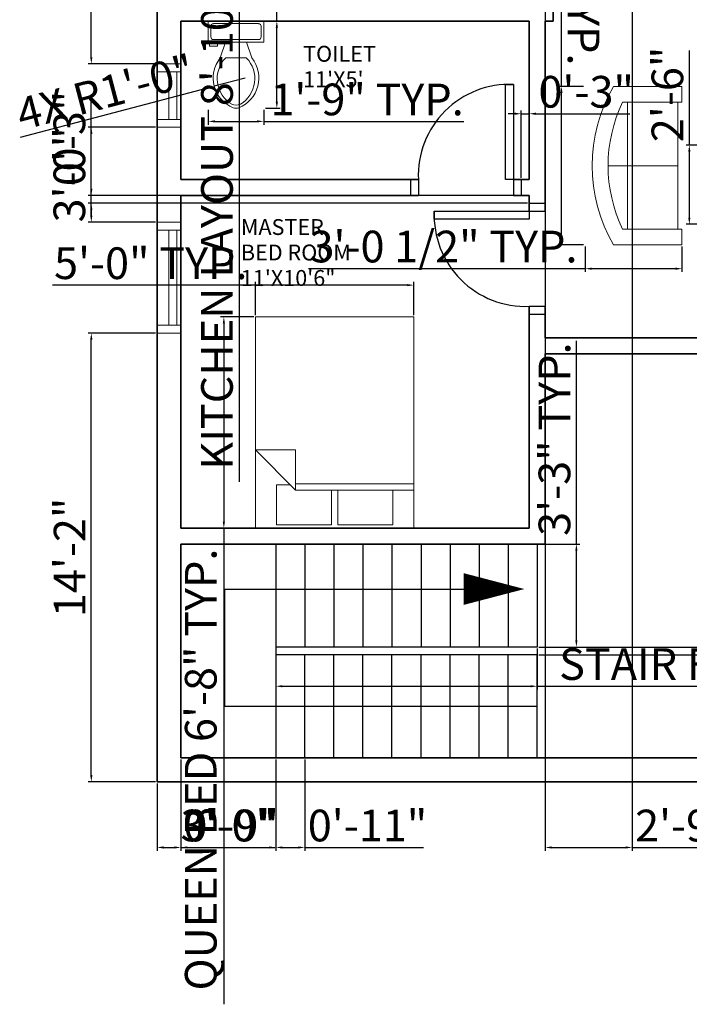
# Model space of a CAD drawing. Units: inches. Extents: x 2330 to 2931, y 514 to 1098.
# Tile 1 of 4: x 2330 to 2583, y 514 to 887. Entities that reach past the tile are written whole.
import ezdxf

# ---------------------------------------------------------------- set-up
doc = ezdxf.new("R2010")
doc.units = ezdxf.units.IN
for name, color, linetype, lineweight in [('A-ANNO-DIMS', 2, 'Continuous', 18), ('A-AREA-IDEN', 7, 'Continuous', 18), ('A-DOOR', 3, 'Continuous', 25), ('A-FLOR-FIXT', 9, 'Continuous', 18), ('A-FLOR-STRS', 7, 'Continuous', 25), ('A-FURN', 8, 'Continuous', 18), ('A-GLAZ', 4, 'Continuous', 18), ('A-WALL', 7, 'Continuous', 35)]:
    doc.layers.add(name, color=color, linetype=linetype, lineweight=lineweight)
doc.styles.get("Standard").update_dxf_attribs({"font": 'arial.ttf'})
doc.dimstyles.new('ISO-25', dxfattribs={"dimtxt": 12, "dimasz": 2.5, "dimexe": 1.25, "dimexo": 0.625, "dimtad": 1, "dimdec": 1, "dimlunit": 3, "dimtxsty": 'Standard', "dimcen": 2.5, "dimadec": 0, "dimazin": 0, "dimtfac": 1, "dimtdec": 1, "dimtmove": 0, "dimatfit": 3, "dimfxl": 1, "dimarcsym": 0})

# ---------------------------------------------------------------- blocks, each defined once
blk = doc.blocks.new('Toilet - top')
for p, q in [((9.5, -6), (9.5, -2)), ((-10, -8.5), (-8, -8.5)), ((-10, -9.5), (-10, -8.5)), ((-7, -9.5), (-10, -9.5)), ((-8, -8.5), (-8, -8)), ((-7, -8), (-7, -9.5)), ((-4, -8), (-6, -14)), ((4, -8), (6, -14)), ((4, -14), (-4, -14))]:
    blk.add_line(p, q)
blk.add_lwpolyline([(10.5, -8), (10.5, 0), (-10.5, 0), (-10.5, -8)], close=True)
for points in [[(-9.5, -2), (-9.5, -6)], [(8.5, -1), (-8.5, -1)], [(-8.5, -7), (8.5, -7)]]:
    blk.add_lwpolyline(points)
for centre, radius, start, end in [((-8.62, -1.88), 0.884, 81.8699, 188.1301), ((8.62, -1.88), 0.884, 351.8699, 98.1301), ((-8.62, -6.12), 0.884, 171.8699, 278.1301), ((8.62, -6.12), 0.884, 261.8699, 8.1301), ((3.52, -21.58), 12.17, 141.4691, 247.9714), ((4.2, -21.82), 11.33, 136.3677, 238.9468), ((-3.52, -21.58), 12.17, 292.0284, 38.5307), ((-4.2, -21.82), 11.33, 301.053, 43.6321), ((0, -27.88), 4, 245.7318, 294.2682), ((0, -29), 4, 254.8605, 285.1395)]:
    blk.add_arc(centre, radius, start, end)
blk = doc.blocks.new('Bed - Queen')
for p, q in [((0, -80.00003), (0, 0)), ((0, 0), (59.99999, 0)), ((59.99999, 0), (59.99999, -80.00003)), ((7.99999, -1.2), (28.79998, -1.2)), ((7.99999, -14.4), (7.99999, -1.2)), ((28.79998, -1.2), (28.79998, -14.4)), ((31.19999, -1.2), (51.99999, -1.2)), ((31.19999, -14.4), (31.19999, -1.2)), ((51.99999, -1.2), (51.99999, -16.4)), ((0, -14.4), (44.8, -14.4)), ((59.99999, -29.6), (44.8, -14.4)), ((44.8, -14.4), (44.8, -29.6)), ((44.8, -16.8), (0, -16.8)), ((51.99999, -16.4), (46.79936, -16.4)), ((44.8, -29.6), (59.99999, -29.6)), ((59.99999, -80.00003), (0, -80.00003))]:
    blk.add_line(p, q)
blk = doc.blocks.new('Sofa - Roundback Loveseat 5 ft.')
for p, q in [((0, -32.44198), (0, -5.99998)), ((-24, -33.99998), (-24, -11.46958)), ((-23.9998, -13.38178), (23.99986, -13.38178)), ((24.00004, -33.99998), (24.00004, -11.46958)), ((-24, -32.44198), (24.00004, -32.44198))]:
    blk.add_line(p, q)
for points in [[(-24, -33.99998), (-30, -33.99998), (-30, -7.99998)], [(30.00004, -7.99998), (30.00004, -33.99998), (24.00004, -33.99998)]]:
    blk.add_lwpolyline(points)
for centre, radius, start, end in [((0, -60.24998), 60.24998, 60.13715, 119.8628), ((0, -61.38438), 55.38444, 64.32083, 115.6792)]:
    blk.add_arc(centre, radius, start, end)
blk = doc.blocks.new('DOOR-SWING-36IN')
for p, q in [((0, 6), (0, 0)), ((3, 6), (3, 0)), ((39, 6), (39, 0)), ((42, 6), (42, 0))]:
    blk.add_line(p, q)
blk.add_lwpolyline([(39, 6), (36, 6), (36, 42), (39, 42)], close=True)
blk.add_arc((37.5, 7.5), 34.53, 87.5104, 182.4896)
blk = doc.blocks.new('WIN-36IN')
for p, q in [((0, 9), (0, 0)), ((39, 9), (3, 9)), ((3, 9), (3, 0)), ((39, 0), (39, 9)), ((42, 0), (42, 9)), ((3, 4.5), (39, 4.5)), ((3, 1.5), (39, 1.5)), ((3, 0), (39, 0))]:
    blk.add_line(p, q)
blk = doc.blocks.new('WIN-18IN')
for p, q in [((0, 9), (0, 0)), ((21, 9), (3, 9)), ((3, 9), (3, 0)), ((21, 0), (21, 9)), ((24, 0), (24, 9)), ((3, 4.5), (21, 4.5)), ((3, 1.5), (21, 1.5)), ((3, 0), (21, 0))]:
    blk.add_line(p, q)
blk = doc.blocks.new('STAIR-FLIGHT-9-TREAD')
for p, q in [((11, 39), (11, 0)), ((22, 39), (22, 0)), ((33, 39), (33, 0)), ((44, 39), (44, 0)), ((55, 39), (55, 0)), ((66, 39), (66, 0)), ((77, 39), (77, 0)), ((88, 39), (88, 0)), ((99, 39), (99, 0)), ((99, 0), (0, 0))]:
    blk.add_line(p, q)
blk = doc.blocks.new('*D21')
at = {"layer": 'A-ANNO-DIMS', "color": 0, "lineweight": -2, "transparency": 16777216}
for p, q in [((2418.49, 774.47), (2405.87, 774.47)), ((2407.12, 771.97), (2407.12, 696.97)), ((2418.49, 694.47), (2405.87, 694.47)), ((2407.12, 694.47), (2407.12, 514.2))]:
    blk.add_line(p, q, dxfattribs=at)
at = {"layer": 'A-ANNO-DIMS', "color": 0, "transparency": 16777216}
for points in [[(2406.7, 771.97), (2407.53, 771.97), (2407.12, 774.47)], [(2406.7, 696.97), (2407.53, 696.97), (2407.12, 694.47)]]:
    blk.add_solid(points, dxfattribs=at)
at = {"layer": 'Defpoints', "color": 0, "transparency": 16777216}
for p in [(2419.12, 774.47), (2407.12, 694.47), (2419.12, 694.47)]:
    blk.add_point(p, dxfattribs=at)
at = {"layer": 'A-ANNO-DIMS', "color": 0, "transparency": 16777216, "insert": (2399.92, 603.09), "char_height": 12, "attachment_point": 5, "rotation": 90}
blk.add_mtext('QUEEN BED 6\'-8" TYP.', dxfattribs=at)
blk = doc.blocks.new('*D22')
at = {"layer": 'A-ANNO-DIMS', "color": 0, "lineweight": -2, "transparency": 16777216}
for p, q in [((2419.12, 775.1), (2419.12, 787.72)), ((2479.12, 775.1), (2479.12, 787.72)), ((2419.12, 786.47), (2342.22, 786.47)), ((2476.62, 786.47), (2421.62, 786.47))]:
    blk.add_line(p, q, dxfattribs=at)
at = {"layer": 'A-ANNO-DIMS', "color": 0, "transparency": 16777216}
for points in [[(2421.62, 786.89), (2421.62, 786.06), (2419.12, 786.47)], [(2476.62, 786.89), (2476.62, 786.06), (2479.12, 786.47)]]:
    blk.add_solid(points, dxfattribs=at)
at = {"layer": 'Defpoints', "color": 0, "transparency": 16777216}
for p in [(2419.12, 786.47), (2419.12, 774.47), (2479.12, 774.47)]:
    blk.add_point(p, dxfattribs=at)
at = {"layer": 'A-ANNO-DIMS', "color": 0, "transparency": 16777216, "insert": (2379.42, 793.22), "char_height": 12, "attachment_point": 5}
blk.add_mtext('5\'-0" TYP.', dxfattribs=at)
blk = doc.blocks.new('*D23')
at = {"layer": 'A-ANNO-DIMS', "color": 0, "lineweight": -2, "transparency": 16777216}
for p, q in [((2427.19, 886.47), (2427.19, 996.45)), ((2422.86, 886.47), (2428.44, 886.47)), ((2427.19, 855.93), (2427.19, 883.97)), ((2422.86, 853.43), (2428.44, 853.43))]:
    blk.add_line(p, q, dxfattribs=at)
at = {"layer": 'A-ANNO-DIMS', "color": 0, "transparency": 16777216}
for points in [[(2426.77, 883.97), (2427.61, 883.97), (2427.19, 886.47)], [(2426.77, 855.93), (2427.61, 855.93), (2427.19, 853.43)]]:
    blk.add_solid(points, dxfattribs=at)
at = {"layer": 'Defpoints', "color": 0, "transparency": 16777216}
for p in [(2422.23, 886.47), (2427.19, 886.47), (2422.23, 853.43)]:
    blk.add_point(p, dxfattribs=at)
at = {"layer": 'A-ANNO-DIMS', "color": 0, "transparency": 16777216, "insert": (2420.36, 942.71), "char_height": 12, "attachment_point": 5, "rotation": 90}
blk.add_mtext('WC 2\'-9" TYP.', dxfattribs=at)
blk = doc.blocks.new('*D24')
at = {"layer": 'A-ANNO-DIMS', "color": 0, "lineweight": -2, "transparency": 16777216}
for p, q in [((2401.23, 852.8), (2401.23, 847.22)), ((2422.23, 852.8), (2422.23, 847.22)), ((2403.73, 848.47), (2419.73, 848.47)), ((2422.23, 848.47), (2498, 848.47))]:
    blk.add_line(p, q, dxfattribs=at)
at = {"layer": 'A-ANNO-DIMS', "color": 0, "transparency": 16777216}
for points in [[(2403.73, 848.89), (2403.73, 848.05), (2401.23, 848.47)], [(2419.73, 848.89), (2419.73, 848.05), (2422.23, 848.47)]]:
    blk.add_solid(points, dxfattribs=at)
at = {"layer": 'Defpoints', "color": 0, "transparency": 16777216}
for p in [(2401.23, 853.43), (2422.23, 853.43), (2422.23, 848.47)]:
    blk.add_point(p, dxfattribs=at)
at = {"layer": 'A-ANNO-DIMS', "color": 0, "transparency": 16777216, "insert": (2461.36, 855.22), "char_height": 12, "attachment_point": 5}
blk.add_mtext('1\'-9" TYP.', dxfattribs=at)
blk = doc.blocks.new('*D25')
at = {"layer": 'A-ANNO-DIMS', "color": 0, "lineweight": -2, "transparency": 16777216}
for p, q in [((2535, 861.7), (2535, 1031.23)), ((2543.37, 861.7), (2533.75, 861.7)), ((2535, 804.2), (2535, 859.2)), ((2543.37, 801.7), (2533.75, 801.7))]:
    blk.add_line(p, q, dxfattribs=at)
at = {"layer": 'A-ANNO-DIMS', "color": 0, "transparency": 16777216}
for points in [[(2535.41, 859.2), (2534.58, 859.2), (2535, 861.7)], [(2535.41, 804.2), (2534.58, 804.2), (2535, 801.7)]]:
    blk.add_solid(points, dxfattribs=at)
at = {"layer": 'Defpoints', "color": 0, "transparency": 16777216}
for p in [(2535, 861.7), (2544, 861.7), (2544, 801.7)]:
    blk.add_point(p, dxfattribs=at)
at = {"layer": 'A-ANNO-DIMS', "color": 0, "transparency": 16777216, "insert": (2541.83, 947.72), "char_height": 12, "attachment_point": 5, "rotation": 270.0001}
blk.add_mtext('LOVESEAT 5\'-0" TYP.', dxfattribs=at)
blk = doc.blocks.new('*D26')
at = {"layer": 'A-ANNO-DIMS', "color": 0, "lineweight": -2, "transparency": 16777216}
for p, q in [((2544, 801.08), (2544, 791.45)), ((2580.66, 801.08), (2580.66, 791.45)), ((2544, 792.7), (2439.15, 792.7)), ((2578.16, 792.7), (2546.5, 792.7))]:
    blk.add_line(p, q, dxfattribs=at)
at = {"layer": 'A-ANNO-DIMS', "color": 0, "transparency": 16777216}
for points in [[(2546.5, 793.12), (2546.5, 792.28), (2544, 792.7)], [(2578.16, 793.12), (2578.16, 792.28), (2580.66, 792.7)]]:
    blk.add_solid(points, dxfattribs=at)
at = {"layer": 'Defpoints', "color": 0, "transparency": 16777216}
for p in [(2544, 801.7), (2580.66, 801.7), (2544, 792.7)]:
    blk.add_point(p, dxfattribs=at)
at = {"layer": 'A-ANNO-DIMS', "color": 0, "transparency": 16777216, "insert": (2490.32, 799.53), "char_height": 12, "attachment_point": 5, "rotation": 0.0001}
blk.add_mtext('3\'-0 1/2" TYP.', dxfattribs=at)
blk = doc.blocks.new('*D29')
at = {"layer": 'A-ANNO-DIMS', "color": 0, "lineweight": -2, "transparency": 16777216}
for p, q in [((2426.8, 648.85), (2426.8, 633.37)), ((2525.8, 648.85), (2525.8, 633.37)), ((2429.3, 634.62), (2523.3, 634.62)), ((2525.8, 634.62), (2720.93, 634.62))]:
    blk.add_line(p, q, dxfattribs=at)
at = {"layer": 'A-ANNO-DIMS', "color": 0, "transparency": 16777216}
for points in [[(2429.3, 635.04), (2429.3, 634.21), (2426.8, 634.62)], [(2523.3, 635.04), (2523.3, 634.21), (2525.8, 634.62)]]:
    blk.add_solid(points, dxfattribs=at)
at = {"layer": 'Defpoints', "color": 0, "transparency": 16777216}
for p in [(2426.8, 649.47), (2525.8, 649.47), (2525.8, 634.62)]:
    blk.add_point(p, dxfattribs=at)
at = {"layer": 'A-ANNO-DIMS', "color": 0, "transparency": 16777216, "insert": (2624.62, 641.46), "char_height": 12, "attachment_point": 5}
blk.add_mtext('STAIR FLIGHT 8\'-3" TYP.', dxfattribs=at)
blk = doc.blocks.new('*D30')
at = {"layer": 'A-ANNO-DIMS', "color": 0, "lineweight": -2, "transparency": 16777216}
for p, q in [((2540.65, 688.47), (2540.65, 765.36)), ((2526.43, 688.47), (2541.9, 688.47)), ((2540.65, 651.97), (2540.65, 685.97)), ((2526.43, 649.47), (2541.9, 649.47))]:
    blk.add_line(p, q, dxfattribs=at)
at = {"layer": 'A-ANNO-DIMS', "color": 0, "transparency": 16777216}
for points in [[(2540.24, 685.97), (2541.07, 685.97), (2540.65, 688.47)], [(2540.24, 651.97), (2541.07, 651.97), (2540.65, 649.47)]]:
    blk.add_solid(points, dxfattribs=at)
at = {"layer": 'Defpoints', "color": 0, "transparency": 16777216}
for p in [(2525.8, 688.47), (2540.65, 688.47), (2525.8, 649.47)]:
    blk.add_point(p, dxfattribs=at)
at = {"layer": 'A-ANNO-DIMS', "color": 0, "transparency": 16777216, "insert": (2533.9, 728.17), "char_height": 12, "attachment_point": 5, "rotation": 90}
blk.add_mtext('3\'-3" TYP.', dxfattribs=at)
blk = doc.blocks.new('*D31')
at = {"layer": 'A-ANNO-DIMS', "color": 0, "lineweight": -2, "transparency": 16777216}
for p, q in [((2428.18, 1012.47), (2411.65, 1012.47)), ((2412.9, 1009.97), (2412.9, 908.97)), ((2428.18, 906.47), (2411.65, 906.47)), ((2412.9, 906.47), (2412.9, 712.06))]:
    blk.add_line(p, q, dxfattribs=at)
at = {"layer": 'A-ANNO-DIMS', "color": 0, "transparency": 16777216}
for points in [[(2412.49, 1009.97), (2413.32, 1009.97), (2412.9, 1012.47)], [(2412.49, 908.97), (2413.32, 908.97), (2412.9, 906.47)]]:
    blk.add_solid(points, dxfattribs=at)
at = {"layer": 'Defpoints', "color": 0, "transparency": 16777216}
for p in [(2428.8, 1012.47), (2412.9, 906.47), (2428.8, 906.47)]:
    blk.add_point(p, dxfattribs=at)
at = {"layer": 'A-ANNO-DIMS', "color": 0, "transparency": 16777216, "insert": (2406.07, 808.02), "char_height": 12, "attachment_point": 5, "rotation": 90}
blk.add_mtext('KITCHEN LAYOUT 8\'-10"', dxfattribs=at)
blk = doc.blocks.new('*D34')
at = {"layer": 'A-ANNO-DIMS', "color": 0, "lineweight": -2, "transparency": 16777216}
for p, q in [((2583.44, 839.51), (2583.44, 875.36)), ((2591.82, 839.51), (2582.19, 839.51)), ((2583.44, 812.01), (2583.44, 837.01)), ((2591.82, 809.51), (2582.19, 809.51))]:
    blk.add_line(p, q, dxfattribs=at)
at = {"layer": 'A-ANNO-DIMS', "color": 0, "transparency": 16777216}
for points in [[(2583.03, 837.01), (2583.86, 837.01), (2583.44, 839.51)], [(2583.03, 812.01), (2583.86, 812.01), (2583.44, 809.51)]]:
    blk.add_solid(points, dxfattribs=at)
at = {"layer": 'Defpoints', "color": 0, "transparency": 16777216}
for p in [(2583.44, 839.51), (2592.44, 839.51), (2592.44, 809.51)]:
    blk.add_point(p, dxfattribs=at)
at = {"layer": 'A-ANNO-DIMS', "color": 0, "transparency": 16777216, "insert": (2576.69, 858.69), "char_height": 12, "attachment_point": 5, "rotation": 90}
blk.add_mtext('2\'-6"', dxfattribs=at)
blk = doc.blocks.new('*D42')
at = {"layer": 'A-ANNO-DIMS', "color": 0, "lineweight": -2, "transparency": 16777216}
for p, q in [((2381.18, 768.34), (2355.66, 768.34)), ((2356.91, 600.97), (2356.91, 765.84)), ((2381.18, 598.47), (2355.66, 598.47))]:
    blk.add_line(p, q, dxfattribs=at)
at = {"layer": 'A-ANNO-DIMS', "color": 0, "transparency": 16777216}
for points in [[(2356.49, 765.84), (2357.33, 765.84), (2356.91, 768.34)], [(2356.49, 600.97), (2357.33, 600.97), (2356.91, 598.47)]]:
    blk.add_solid(points, dxfattribs=at)
at = {"layer": 'Defpoints', "color": 0, "transparency": 16777216}
for p in [(2356.91, 768.34), (2381.8, 768.34), (2381.8, 598.47)]:
    blk.add_point(p, dxfattribs=at)
at = {"layer": 'A-ANNO-DIMS', "color": 0, "transparency": 16777216, "insert": (2350.26, 683.41), "char_height": 12, "attachment_point": 5, "rotation": 90}
blk.add_mtext('14\'-2"', dxfattribs=at)
blk = doc.blocks.new('*D43')
at = {"layer": 'A-ANNO-DIMS', "color": 0, "lineweight": -2, "transparency": 16777216}
for p, q in [((2381.18, 846.23), (2355.66, 846.23)), ((2356.91, 812.84), (2356.91, 843.73)), ((2381.18, 810.34), (2355.66, 810.34))]:
    blk.add_line(p, q, dxfattribs=at)
at = {"layer": 'A-ANNO-DIMS', "color": 0, "transparency": 16777216}
for points in [[(2356.49, 843.73), (2357.33, 843.73), (2356.91, 846.23)], [(2356.49, 812.84), (2357.33, 812.84), (2356.91, 810.34)]]:
    blk.add_solid(points, dxfattribs=at)
at = {"layer": 'Defpoints', "color": 0, "transparency": 16777216}
for p in [(2356.91, 846.23), (2381.8, 846.23), (2381.8, 810.34)]:
    blk.add_point(p, dxfattribs=at)
at = {"layer": 'A-ANNO-DIMS', "color": 0, "transparency": 16777216, "insert": (2350.15, 828.29), "char_height": 12, "attachment_point": 5, "rotation": 90}
blk.add_mtext('3\'-0"', dxfattribs=at)
blk = doc.blocks.new('*D44')
at = {"layer": 'A-ANNO-DIMS', "color": 0, "lineweight": -2, "transparency": 16777216}
for p, q in [((2356.91, 892.47), (2356.91, 936.31)), ((2390.18, 892.47), (2355.66, 892.47)), ((2356.91, 872.73), (2356.91, 889.97)), ((2381.18, 870.23), (2355.66, 870.23))]:
    blk.add_line(p, q, dxfattribs=at)
at = {"layer": 'A-ANNO-DIMS', "color": 0, "transparency": 16777216}
for points in [[(2356.49, 889.97), (2357.33, 889.97), (2356.91, 892.47)], [(2356.49, 872.73), (2357.33, 872.73), (2356.91, 870.23)]]:
    blk.add_solid(points, dxfattribs=at)
at = {"layer": 'Defpoints', "color": 0, "transparency": 16777216}
for p in [(2356.91, 892.47), (2390.8, 892.47), (2381.8, 870.23)]:
    blk.add_point(p, dxfattribs=at)
at = {"layer": 'A-ANNO-DIMS', "color": 0, "transparency": 16777216, "insert": (2350.16, 915.64), "char_height": 12, "attachment_point": 5, "rotation": 90}
blk.add_mtext('1\'-10"', dxfattribs=at)
blk = doc.blocks.new('*D48')
at = {"layer": 'A-ANNO-DIMS', "color": 0, "lineweight": -2, "transparency": 16777216}
for p, q in [((2390.8, 606.85), (2390.8, 572.33)), ((2426.8, 606.85), (2426.8, 572.33)), ((2393.3, 573.58), (2424.3, 573.58))]:
    blk.add_line(p, q, dxfattribs=at)
at = {"layer": 'A-ANNO-DIMS', "color": 0, "transparency": 16777216}
for points in [[(2393.3, 574), (2393.3, 573.16), (2390.8, 573.58)], [(2424.3, 574), (2424.3, 573.16), (2426.8, 573.58)]]:
    blk.add_solid(points, dxfattribs=at)
at = {"layer": 'Defpoints', "color": 0, "transparency": 16777216}
for p in [(2390.8, 607.47), (2426.8, 607.47), (2426.8, 573.58)]:
    blk.add_point(p, dxfattribs=at)
at = {"layer": 'A-ANNO-DIMS', "color": 0, "transparency": 16777216, "insert": (2408.8, 580.34), "char_height": 12, "attachment_point": 5}
blk.add_mtext('3\'-0"', dxfattribs=at)
blk = doc.blocks.new('*D49')
at = {"layer": 'A-ANNO-DIMS', "color": 0, "lineweight": -2, "transparency": 16777216}
for p, q in [((2390.8, 606.85), (2390.8, 572.33)), ((2381.8, 597.85), (2381.8, 572.33)), ((2384.3, 573.58), (2388.3, 573.58)), ((2390.8, 573.58), (2426.45, 573.58))]:
    blk.add_line(p, q, dxfattribs=at)
at = {"layer": 'A-ANNO-DIMS', "color": 0, "transparency": 16777216}
for points in [[(2384.3, 574), (2384.3, 573.16), (2381.8, 573.58)], [(2388.3, 574), (2388.3, 573.16), (2390.8, 573.58)]]:
    blk.add_solid(points, dxfattribs=at)
at = {"layer": 'Defpoints', "color": 0, "transparency": 16777216}
for p in [(2390.8, 607.47), (2381.8, 598.47), (2390.8, 573.58)]:
    blk.add_point(p, dxfattribs=at)
at = {"layer": 'A-ANNO-DIMS', "color": 0, "transparency": 16777216, "insert": (2409.88, 580.33), "char_height": 12, "attachment_point": 5}
blk.add_mtext('0\'-9"', dxfattribs=at)
blk = doc.blocks.new('*D50')
at = {"layer": 'A-ANNO-DIMS', "color": 0, "lineweight": -2, "transparency": 16777216}
for p, q in [((2426.8, 606.85), (2426.8, 572.33)), ((2437.8, 606.85), (2437.8, 572.33)), ((2429.3, 573.58), (2435.3, 573.58)), ((2437.8, 573.58), (2482.78, 573.58))]:
    blk.add_line(p, q, dxfattribs=at)
at = {"layer": 'A-ANNO-DIMS', "color": 0, "transparency": 16777216}
for points in [[(2429.3, 574), (2429.3, 573.16), (2426.8, 573.58)], [(2435.3, 574), (2435.3, 573.16), (2437.8, 573.58)]]:
    blk.add_solid(points, dxfattribs=at)
at = {"layer": 'Defpoints', "color": 0, "transparency": 16777216}
for p in [(2426.8, 607.47), (2437.8, 607.47), (2437.8, 573.58)]:
    blk.add_point(p, dxfattribs=at)
at = {"layer": 'A-ANNO-DIMS', "color": 0, "transparency": 16777216, "insert": (2461.54, 580.33), "char_height": 12, "attachment_point": 5}
blk.add_mtext('0\'-11"', dxfattribs=at)
blk = doc.blocks.new('*D52')
at = {"layer": 'A-ANNO-DIMS', "color": 0, "lineweight": -2, "transparency": 16777216}
for p, q in [((2778.7, 651.97), (2778.7, 687.62)), ((2526.43, 649.47), (2779.95, 649.47)), ((2778.7, 646.47), (2778.7, 649.47)), ((2526.43, 646.47), (2779.95, 646.47)), ((2778.7, 643.97), (2778.7, 641.47))]:
    blk.add_line(p, q, dxfattribs=at)
at = {"layer": 'A-ANNO-DIMS', "color": 0, "transparency": 16777216}
for points in [[(2778.28, 651.97), (2779.11, 651.97), (2778.7, 649.47)], [(2778.28, 643.97), (2779.11, 643.97), (2778.7, 646.47)]]:
    blk.add_solid(points, dxfattribs=at)
at = {"layer": 'Defpoints', "color": 0, "transparency": 16777216}
for p in [(2525.8, 649.47), (2778.7, 649.47), (2525.8, 646.47)]:
    blk.add_point(p, dxfattribs=at)
at = {"layer": 'A-ANNO-DIMS', "color": 0, "transparency": 16777216, "insert": (2771.94, 671.05), "char_height": 12, "attachment_point": 5, "rotation": 90}
blk.add_mtext('0\'-3"', dxfattribs=at)
blk = doc.blocks.new('*D54')
at = {"layer": 'A-ANNO-DIMS', "color": 0, "lineweight": -2, "transparency": 16777216}
for p, q in [((2517.3, 851.36), (2514.8, 851.36)), ((2519.8, 827.1), (2519.8, 852.61)), ((2519.8, 851.36), (2522.8, 851.36)), ((2522.8, 827.1), (2522.8, 852.61)), ((2525.3, 851.36), (2560.95, 851.36))]:
    blk.add_line(p, q, dxfattribs=at)
at = {"layer": 'A-ANNO-DIMS', "color": 0, "transparency": 16777216}
for points in [[(2517.3, 851.78), (2517.3, 850.95), (2519.8, 851.36)], [(2525.3, 851.78), (2525.3, 850.95), (2522.8, 851.36)]]:
    blk.add_solid(points, dxfattribs=at)
at = {"layer": 'Defpoints', "color": 0, "transparency": 16777216}
for p in [(2522.8, 851.36), (2519.8, 826.47), (2522.8, 826.47)]:
    blk.add_point(p, dxfattribs=at)
at = {"layer": 'A-ANNO-DIMS', "color": 0, "transparency": 16777216, "insert": (2544.38, 858.12), "char_height": 12, "attachment_point": 5}
blk.add_mtext('0\'-3"', dxfattribs=at)
blk = doc.blocks.new('*D55')
at = {"layer": 'A-ANNO-DIMS', "color": 0, "lineweight": -2, "transparency": 16777216}
for p, q in [((2356.91, 822.97), (2356.91, 858.62)), ((2522.18, 820.47), (2355.66, 820.47)), ((2356.91, 817.47), (2356.91, 820.47)), ((2522.18, 817.47), (2355.66, 817.47)), ((2356.91, 814.97), (2356.91, 812.47))]:
    blk.add_line(p, q, dxfattribs=at)
at = {"layer": 'A-ANNO-DIMS', "color": 0, "transparency": 16777216}
for points in [[(2356.49, 822.97), (2357.33, 822.97), (2356.91, 820.47)], [(2356.49, 814.97), (2357.33, 814.97), (2356.91, 817.47)]]:
    blk.add_solid(points, dxfattribs=at)
at = {"layer": 'Defpoints', "color": 0, "transparency": 16777216}
for p in [(2356.91, 820.47), (2522.8, 820.47), (2522.8, 817.47)]:
    blk.add_point(p, dxfattribs=at)
at = {"layer": 'A-ANNO-DIMS', "color": 0, "transparency": 16777216, "insert": (2350.15, 842.05), "char_height": 12, "attachment_point": 5, "rotation": 90}
blk.add_mtext('0\'-3"', dxfattribs=at)
blk = doc.blocks.new('*D56')
at = {"layer": 'A-ANNO-DIMS', "color": 0, "lineweight": -2, "transparency": 16777216}
for p, q in [((2528.8, 945.85), (2528.8, 572.33)), ((2561.8, 945.85), (2561.8, 572.33)), ((2531.3, 573.58), (2559.3, 573.58)), ((2561.8, 573.58), (2597.66, 573.58))]:
    blk.add_line(p, q, dxfattribs=at)
at = {"layer": 'A-ANNO-DIMS', "color": 0, "transparency": 16777216}
for points in [[(2531.3, 574), (2531.3, 573.16), (2528.8, 573.58)], [(2559.3, 574), (2559.3, 573.16), (2561.8, 573.58)]]:
    blk.add_solid(points, dxfattribs=at)
at = {"layer": 'Defpoints', "color": 0, "transparency": 16777216}
for p in [(2528.8, 946.47), (2561.8, 946.47), (2561.8, 573.58)]:
    blk.add_point(p, dxfattribs=at)
at = {"layer": 'A-ANNO-DIMS', "color": 0, "transparency": 16777216, "insert": (2580.98, 580.33), "char_height": 12, "attachment_point": 5}
blk.add_mtext('2\'-9"', dxfattribs=at)
blk = doc.blocks.new('*D63')
at = {"layer": 'A-ANNO-DIMS', "color": 0, "lineweight": -2, "transparency": 16777216}
for p, q in [((2415.25, 864.89), (2403.48, 861.8)), ((2330.07, 842.52), (2401.06, 861.16))]:
    blk.add_line(p, q, dxfattribs=at)
at = {"layer": 'A-ANNO-DIMS', "color": 0, "transparency": 16777216}
blk.add_solid([(2400.96, 861.57), (2401.17, 860.76), (2403.48, 861.8)], dxfattribs=at)
at = {"layer": 'Defpoints', "color": 0, "transparency": 16777216}
for p in [(2415.25, 864.89), (2403.48, 861.8)]:
    blk.add_point(p, dxfattribs=at)
at = {"layer": 'A-ANNO-DIMS', "color": 0, "transparency": 16777216, "insert": (2362.64, 858.05), "char_height": 12, "attachment_point": 5, "rotation": 14.7175}
blk.add_mtext('4X R1\'-0"', dxfattribs=at)

msp = doc.modelspace()

# ---------------------------------------------------------------- linework, layer by layer
at = {"layer": 'A-FLOR-STRS'}
msp.add_line((2426.8, 688.47), (2426.8, 607.47), dxfattribs=at)
msp.add_lwpolyline([(2497.99, 671.42, 12, 0, 0), (2520.95, 671.42, 0, 0, 0)], format="xyseb", dxfattribs=at)
msp.add_lwpolyline([(2525.8, 626.97), (2407.53, 626.97), (2407.53, 671.42), (2497.99, 671.42)], dxfattribs=at)
at = {"layer": 'A-WALL'}
for p, q in [((2531.8, 892.47), (2531.8, 886.47)), ((2522.8, 886.47), (2390.8, 886.47)), ((2390.8, 886.47), (2390.8, 826.47)), ((2522.8, 886.47), (2522.8, 826.47)), ((2522.8, 886.47), (2522.8, 826.47)), ((2528.8, 886.47), (2528.8, 814.47)), ((2531.8, 886.47), (2528.8, 886.47)), ((2480.8, 826.47), (2390.8, 826.47)), ((2522.8, 826.47), (2516.8, 826.47)), ((2390.8, 820.47), (2390.8, 694.47)), ((2480.8, 820.47), (2390.8, 820.47)), ((2522.8, 820.47), (2516.8, 820.47)), ((2522.8, 820.47), (2522.8, 814.47)), ((2522.8, 820.47), (2522.8, 814.47)), ((2522.8, 778.47), (2522.8, 694.47)), ((2522.8, 778.47), (2522.8, 694.47)), ((2528.8, 778.47), (2528.8, 766.47)), ((2702.8, 766.47), (2528.8, 766.47)), ((2528.8, 760.47), (2528.8, 688.47)), ((2702.8, 760.47), (2528.8, 760.47)), ((2522.8, 694.47), (2390.8, 694.47)), ((2522.8, 688.47), (2390.8, 688.47)), ((2390.8, 688.47), (2390.8, 607.47)), ((2522.8, 688.47), (2528.8, 688.47)), ((2390.8, 607.47), (2624.83, 607.47))]:
    msp.add_line(p, q, dxfattribs=at)
msp.add_lwpolyline([(2738.8, 598.47), (2753.8, 598.47), (2753.8, 1021.47), (2381.8, 1021.47), (2381.8, 598.47), (2624.83, 598.47)], dxfattribs=at)

# ---------------------------------------------------------------- block references
at = {"layer": 'A-DOOR'}
msp.add_blockref('DOOR-SWING-36IN', (2477.8, 820.47), dxfattribs=at)
at = {"layer": 'A-DOOR', "rotation": 90.0000000000012}
msp.add_blockref('DOOR-SWING-36IN', (2528.8, 775.47), dxfattribs=at)
at = {"layer": 'A-FLOR-FIXT'}
msp.add_blockref('Toilet - top', (2411.73, 886.47), dxfattribs=at)
at = {"layer": 'A-FLOR-STRS'}
msp.add_blockref('STAIR-FLIGHT-9-TREAD', (2426.8, 649.47), dxfattribs=at)
at = {"layer": 'A-FLOR-STRS', "extrusion": (0, 0, -1), "zscale": -1, "rotation": 180}
msp.add_blockref('STAIR-FLIGHT-9-TREAD', (-2426.8, 646.47), dxfattribs=at)
at = {"layer": 'A-FURN'}
for name, p, rotation in [('Sofa - Roundback Loveseat 5 ft.', (2546.66, 831.7), 90.00007865497155), ('Bed - Queen', (2479.12, 694.47), 180)]:
    msp.add_blockref(name, p, dxfattribs=dict(at, rotation=rotation))
at = {"layer": 'A-GLAZ'}
for name, p, rotation in [('WIN-18IN', (2390.8, 846.23), 89.99999999999888), ('WIN-36IN', (2390.8, 768.34), 89.99999999999982)]:
    msp.add_blockref(name, p, dxfattribs=dict(at, rotation=rotation))

# ---------------------------------------------------------------- texts
at = {"layer": 'A-AREA-IDEN'}
for s, p in [('TOILET', (2437.16, 871.06)), ("11'X5'", (2437.16, 861.42)), ('MASTER', (2413.56, 805.47)), ('BED ROOM', (2413.56, 795.83)), ('11\'X10\'6"', (2413.56, 786.19))]:
    msp.add_text(s, height=6, dxfattribs=at).set_placement(p)

# ---------------------------------------------------------------- dimensions: what is measured, and where the dimension line sits
at = {"layer": 'A-ANNO-DIMS'}
for base, p1, p2, angle, text, picture, middle in [((2535, 861.7), (2544, 801.7), (2544, 861.7), 90.0001, 'LOVESEAT <> TYP.', '*D25', (2541.83, 947.72)), ((2412.9, 906.47), (2428.8, 1012.47), (2428.8, 906.47), 270, 'KITCHEN LAYOUT <>', '*D31', (2406.07, 808.02)), ((2427.19, 886.47), (2422.23, 853.43), (2422.23, 886.47), 90, 'WC <> TYP.', '*D23', (2420.36, 942.71)), ((2544, 792.7), (2580.66, 801.7), (2544, 801.7), 180.0001, '<> TYP.', '*D26', (2490.32, 799.53)), ((2419.12, 786.47), (2479.12, 774.47), (2419.12, 774.47), 180, '<> TYP.', '*D22', (2379.42, 793.22)), ((2407.12, 694.47), (2419.12, 774.47), (2419.12, 694.47), 270, 'QUEEN BED <> TYP.', '*D21', (2399.92, 603.09)), ((2540.65, 688.47), (2525.8, 649.47), (2525.8, 688.47), 90, '<> TYP.', '*D30', (2533.9, 728.17))]:
    dim = msp.add_linear_dim(base=base, p1=p1, p2=p2, angle=angle, text=text, dimstyle='ISO-25', override={"dimdec": 1, "dimlfac": 1, "dimrnd": 0, "dimzin": 1, "dimdsep": 46, "dimlunit": 4, "dimfrac": 2}, dxfattribs=at)
    dim.commit()
    dim.dimension.update_dxf_attribs({"geometry": picture, "text_midpoint": middle})
for base, p1, p2, picture, middle in [((2561.8, 573.58), (2528.8, 946.47), (2561.8, 946.47), '*D56', (2580.98, 580.33)), ((2522.8, 851.36), (2519.8, 826.47), (2522.8, 826.47), '*D54', (2544.38, 858.12)), ((2390.8, 573.58), (2381.8, 598.47), (2390.8, 607.47), '*D49', (2409.88, 580.33)), ((2426.8, 573.58), (2390.8, 607.47), (2426.8, 607.47), '*D48', (2408.8, 580.34)), ((2437.8, 573.58), (2426.8, 607.47), (2437.8, 607.47), '*D50', (2461.54, 580.33))]:
    dim = msp.add_linear_dim(base=base, p1=p1, p2=p2, dimstyle='ISO-25', override={"dimdec": 1, "dimlfac": 1, "dimrnd": 0, "dimzin": 1, "dimdsep": 46, "dimlunit": 4, "dimfrac": 2}, dxfattribs=at)
    dim.commit()
    dim.dimension.update_dxf_attribs({"geometry": picture, "text_midpoint": middle})
for base, p1, p2, picture, middle in [((2356.91, 892.47), (2381.8, 870.23), (2390.8, 892.47), '*D44', (2350.16, 915.64)), ((2583.44, 839.51), (2592.44, 809.51), (2592.44, 839.51), '*D34', (2576.69, 858.69)), ((2356.91, 820.47), (2522.8, 817.47), (2522.8, 820.47), '*D55', (2350.15, 842.05)), ((2356.91, 846.23), (2381.8, 810.34), (2381.8, 846.23), '*D43', (2350.15, 828.29)), ((2356.91, 768.34), (2381.8, 598.47), (2381.8, 768.34), '*D42', (2350.26, 683.41)), ((2778.7, 649.47), (2525.8, 646.47), (2525.8, 649.47), '*D52', (2771.94, 671.05))]:
    dim = msp.add_linear_dim(base=base, p1=p1, p2=p2, angle=90, dimstyle='ISO-25', override={"dimdec": 1, "dimlfac": 1, "dimrnd": 0, "dimzin": 1, "dimdsep": 46, "dimlunit": 4, "dimfrac": 2}, dxfattribs=at)
    dim.commit()
    dim.dimension.update_dxf_attribs({"geometry": picture, "text_midpoint": middle})
dim = msp.add_radius_dim(center=(2415.25, 864.89), mpoint=(2403.48, 861.8), text='4X <>', dimstyle='ISO-25', override={"dimdec": 1, "dimlfac": 1, "dimrnd": 0, "dimzin": 1, "dimdsep": 46, "dimlunit": 4, "dimfrac": 2}, dxfattribs=at)
dim.commit()
dim.dimension.update_dxf_attribs({"geometry": '*D63', "text_midpoint": (2362.64, 858.05)})
for base, p1, p2, text, picture, middle in [((2422.23, 848.47), (2401.23, 853.43), (2422.23, 853.43), '<> TYP.', '*D24', (2461.36, 855.22)), ((2525.8, 634.62), (2426.8, 649.47), (2525.8, 649.47), 'STAIR FLIGHT <> TYP.', '*D29', (2624.62, 641.46))]:
    dim = msp.add_linear_dim(base=base, p1=p1, p2=p2, text=text, dimstyle='ISO-25', override={"dimdec": 1, "dimlfac": 1, "dimrnd": 0, "dimzin": 1, "dimdsep": 46, "dimlunit": 4, "dimfrac": 2}, dxfattribs=at)
    dim.commit()
    dim.dimension.update_dxf_attribs({"geometry": picture, "text_midpoint": middle})

doc.saveas('drawing.dxf')
